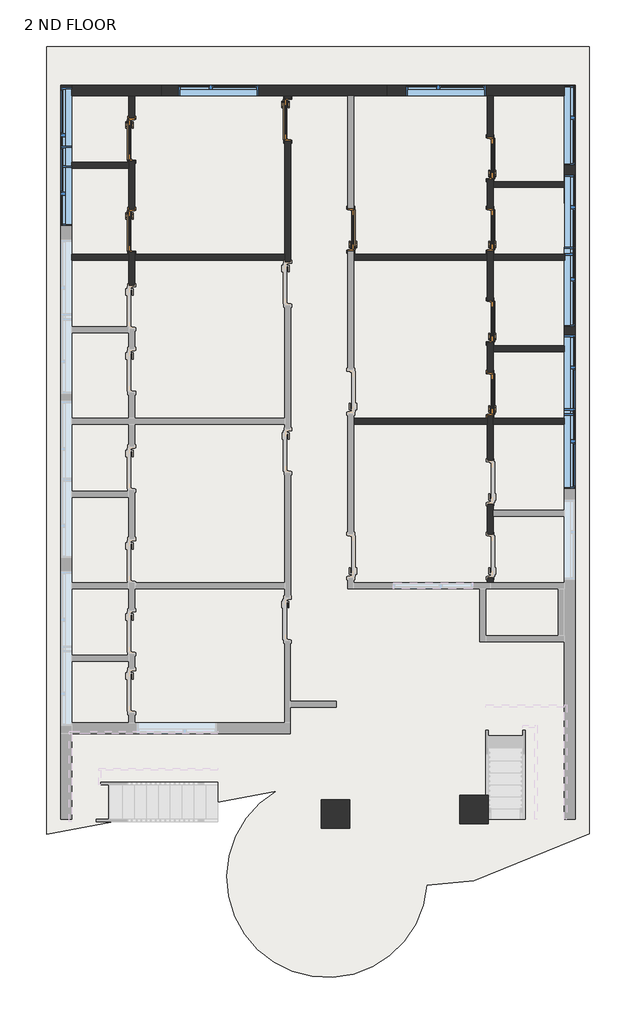
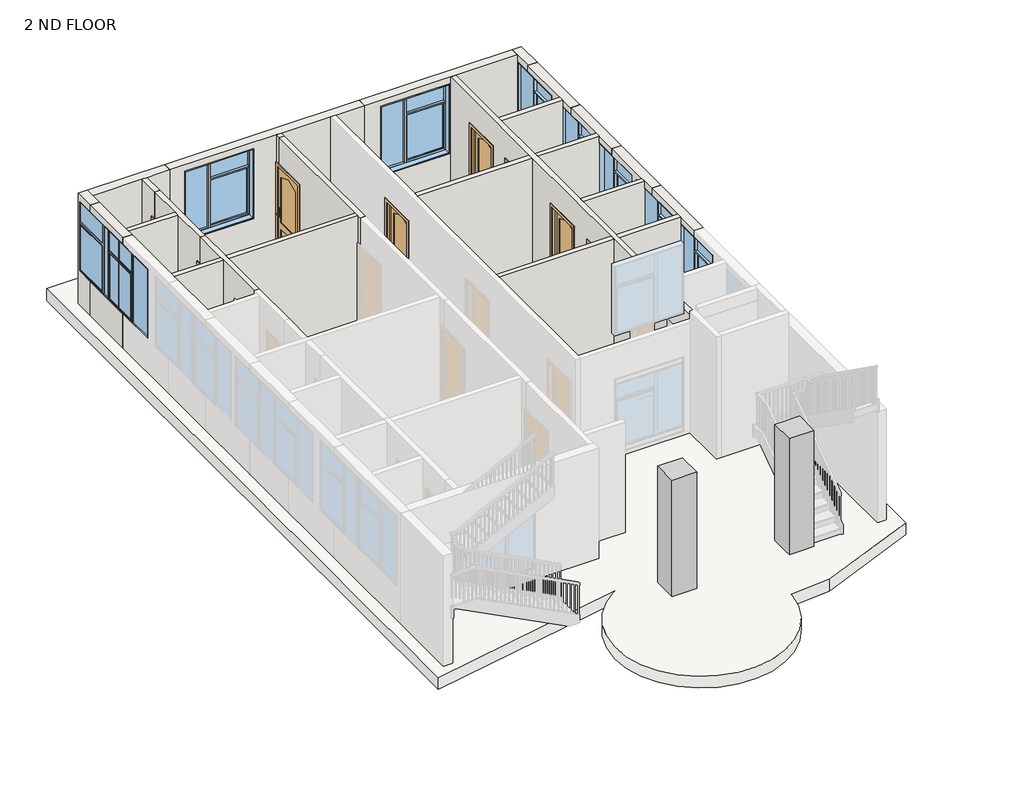
# One storey, part 2 of 4: 25 walls, 9 windows, 8 doors, 2 columns, 1 slab.
"""IFC4 building model written with IfcOpenShell, lengths in millimetres."""

from ifc_helpers import new_model, si_unit, point, frame, frame_2d, origin, place, context, project, spatial, polyline, circle_curve, trimmed, segment, composite_curve, outline, extrude, faceted_brep, transform, mapped, element, save
from components import column_ce31c9ba, door_346b4a94, m_window_casement_double_sidelight_1702_x_1829mm_c8b42c7f

model = new_model("IFC4")

# Units and contexts
model_context = context("Model", 3, world=origin())
ifc_project = project(units=[si_unit("LENGTHUNIT", "METRE", prefix="MILLI")], contexts=[model_context])

# Site, building, storey
site = spatial("IfcSite", under=ifc_project)
building = spatial("IfcBuilding", under=site)
storey = spatial("IfcBuildingStorey", under=building, Name="2 ND FLOOR", Elevation=6400.8)

# Columns
placement = place(None, origin())
element("IfcColumn", 1, ObjectType="Rectangular Column : 24\" x 24\"", at=placement, inside=storey, context=model_context, shape_type="SweptSolid", body=[
    extrude(outline(polyline([(2657.4891134, -7132.8082131), (2657.4891134, -7742.4082131), (2047.8891134, -7742.4082131), (2047.8891134, -7132.8082131), (2657.4891134, -7132.8082131)])), frame((0.0, 0.0, 6400.8), z_axis=(0.0, 0.0, 1.0), x_axis=(1.0, 0.0, 0.0)), (0.0, 0.0, 1.0), 3048.0),
])
column_shape = column_ce31c9ba(model_context)
element("IfcColumn", 2, ObjectType="Rectangular Column : 24\" x 24\"", at=placement, inside=storey, context=model_context, shape_type="MappedRepresentation", body=[
    mapped(column_shape, transform((-606.4108866, -7539.2082131, 0.0), x_axis=(1.0, 0.0, 0.0), y_axis=(0.0, 1.0, 0.0), z_axis=(0.0, 0.0, 1.0))),
])

# Doors
door_shape = door_346b4a94(model_context)
element("IfcDoor", 3, ObjectType="2'10\"X7'", at=placement, inside=storey, context=model_context, shape_type="MappedRepresentation", body=[
    mapped(door_shape, transform((2698.7641134, 6449.4399728, 6400.8), x_axis=(0.0, -1.0, 0.0), y_axis=(1.0, 0.0, 0.0), z_axis=(0.0, 0.0, 1.0))),
])
element("IfcDoor", 4, ObjectType="2'10\"X7'", at=placement, inside=storey, context=model_context, shape_type="MappedRepresentation", body=[
    mapped(door_shape, transform((2698.7641134, 4925.4399728, 6400.8), x_axis=(0.0, -1.0, 0.0), y_axis=(1.0, 0.0, 0.0), z_axis=(0.0, 0.0, 1.0))),
])
element("IfcDoor", 5, ObjectType="2'10\"X7'", at=placement, inside=storey, context=model_context, shape_type="MappedRepresentation", body=[
    mapped(door_shape, transform((2698.7641134, 2969.6399728, 6400.8), x_axis=(0.0, -1.0, 0.0), y_axis=(1.0, 0.0, 0.0), z_axis=(0.0, 0.0, 1.0))),
])
element("IfcDoor", 6, ObjectType="2'10\"X7'", at=placement, inside=storey, context=model_context, shape_type="MappedRepresentation", body=[
    mapped(door_shape, transform((2698.7641134, 1420.2399728, 6400.8), x_axis=(0.0, -1.0, 0.0), y_axis=(1.0, 0.0, 0.0), z_axis=(0.0, 0.0, 1.0))),
])
element("IfcDoor", 7, ObjectType="2'10\"X7'", at=placement, inside=storey, context=model_context, shape_type="MappedRepresentation", body=[
    mapped(door_shape, transform((-273.0358866, 4925.4399728, 6400.8), x_axis=(0.0, -1.0, 0.0), y_axis=(1.0, 0.0, 0.0), z_axis=(0.0, 0.0, 1.0))),
])
element("IfcDoor", 8, ObjectType="2'10\"X7'", at=placement, inside=storey, context=model_context, shape_type="MappedRepresentation", body=[
    mapped(door_shape, transform((-4952.9858866, 4900.320652, 6400.8), x_axis=(0.0, 1.0, 0.0), y_axis=(-1.0, 0.0, 0.0), z_axis=(0.0, 0.0, 1.0))),
])
element("IfcDoor", 9, ObjectType="2'10\"X7'", at=placement, inside=storey, context=model_context, shape_type="MappedRepresentation", body=[
    mapped(door_shape, transform((-4952.9858866, 6843.9929737, 6400.8), x_axis=(0.0, 1.0, 0.0), y_axis=(-1.0, 0.0, 0.0), z_axis=(0.0, 0.0, 1.0))),
])
element("IfcDoor", 10, ObjectType="2'10\"X7'", at=placement, inside=storey, context=model_context, shape_type="MappedRepresentation", body=[
    mapped(door_shape, transform((-1625.5858866, 7274.3310623, 6400.8), x_axis=(0.0, 1.0, 0.0), y_axis=(-1.0, 0.0, 0.0), z_axis=(0.0, 0.0, 1.0))),
])

# Slab
element("IfcSlab", 11, ObjectType="Generic - 12\"", at=placement, inside=storey, context=model_context, shape_type="SweptSolid", body=[
    extrude(outline(composite_curve([segment(polyline([(4815.1311655, 8833.6177996), (4815.1311655, -7955.7822004), (2347.1922936, -8966.8048135), (1347.7141783, -9054.247818)]), True, "CONTINUOUS"), segment(trimmed(circle_curve(frame_2d((-782.1411924, -8888.1832005)), 2136.3195821), [point((1347.7141783, -9054.247818))], [point((-1867.3559444, -7048.0282345))], False, "CARTESIAN"), True, "CONTINUOUS"), segment(polyline([(-1867.3559444, -7048.0282345), (-6765.9108866, -7971.0082131), (-6765.9108866, 8833.6177996), (4815.1311655, 8833.6177996)]), True, "CONTINUOUS")], self_intersect=False)), frame((0.0, 0.0, 6096.0), z_axis=(0.0, 0.0, 1.0), x_axis=(1.0, 0.0, 0.0)), (0.0, 0.0, 1.0), 304.8),
])

# Walls
element("IfcWall", 12, ObjectType="Generic - 4.5\"", at=placement, inside=storey, context=model_context, shape_type="SweptSolid", body=[
    extrude(outline(polyline([(7782.9399728, 9296.4), (7782.9399728, 6400.8), (7300.7929737, 6400.8), (7300.7929737, 8559.4), (7224.9929737, 8559.4), (7224.9929737, 9296.4), (7782.9399728, 9296.4)])), frame((-5013.3108866, 0.0, 0.0), z_axis=(1.0, 0.0, 0.0), x_axis=(0.0, 1.0, 0.0)), (0.0, 0.0, 1.0), 127.0),
])
element("IfcWall", 13, ObjectType="Generic - 4.5\"", at=placement, inside=storey, context=model_context, shape_type="Brep", body=[
    faceted_brep([(-5013.3108866, 5281.320652, 8559.4), (-5013.3108866, 5281.320652, 9296.4), (-5013.3108866, 6233.5399728, 9296.4), (-5013.3108866, 6360.5399728, 9296.4), (-5013.3108866, 7224.9929737, 9296.4), (-5013.3108866, 7224.9929737, 8559.4), (-5013.3108866, 6387.1929737, 8559.4), (-5013.3108866, 6387.1929737, 6400.8), (-5013.3108866, 6360.5399728, 6400.8), (-5013.3108866, 6233.5399728, 6400.8), (-5013.3108866, 5357.120652, 6400.8), (-5013.3108866, 5357.120652, 8559.4), (-4886.3108866, 5281.320652, 9296.4), (-4886.3108866, 5281.320652, 8559.4), (-4886.3108866, 5357.120652, 8559.4), (-4886.3108866, 5357.120652, 6400.8), (-4886.3108866, 6387.1929737, 6400.8), (-4886.3108866, 6387.1929737, 8559.4), (-4886.3108866, 7224.9929737, 8559.4), (-4886.3108866, 7224.9929737, 9296.4)], [[[0, 1, 2, 3, 4, 5, 6, 7, 8, 9, 10, 11]], [[12, 13, 14, 15, 16, 17, 18, 19]], [[15, 10, 9, 8, 7, 16]], [[1, 0, 13, 12]], [[4, 19, 18, 5]], [[14, 11, 10, 15]], [[11, 14, 13, 0]], [[17, 6, 5, 18]], [[6, 17, 16, 7]], [[4, 3, 2, 1, 12, 19]]]),
])
element("IfcWall", 14, ObjectType="Generic - 4.5\"", at=placement, inside=storey, context=model_context, shape_type="SweptSolid", body=[
    extrude(outline(polyline([(-5013.3108866, 6233.5399728), (-6232.5508078, 6233.5399728), (-6232.5508078, 6360.5399728), (-5013.3108866, 6360.5399728), (-5013.3108866, 6233.5399728)])), frame((0.0, 0.0, 6400.8), z_axis=(0.0, 0.0, 1.0), x_axis=(1.0, 0.0, 0.0)), (0.0, 0.0, 1.0), 2895.6),
])
element("IfcWall", 15, ObjectType="Generic - 4.5\"", at=placement, inside=storey, context=model_context, shape_type="SweptSolid", body=[
    extrude(outline(polyline([(-5013.3108866, 4277.7399728), (-6232.5508078, 4277.7399728), (-6232.5508078, 4404.7399728), (-5013.3108866, 4404.7399728), (-5013.3108866, 4277.7399728)])), frame((0.0, 0.0, 6400.8), z_axis=(0.0, 0.0, 1.0), x_axis=(1.0, 0.0, 0.0)), (0.0, 0.0, 1.0), 2895.6),
])
element("IfcWall", 16, ObjectType="Generic - 4.5\"", at=placement, inside=storey, context=model_context, shape_type="Brep", body=[
    faceted_brep([(-5013.3108866, 2968.8174518, 8559.4), (-5013.3108866, 2968.8174518, 9296.4), (-5013.3108866, 4277.7399728, 9296.4), (-5013.3108866, 4404.7399728, 9296.4), (-5013.3108866, 5281.320652, 9296.4), (-5013.3108866, 5281.320652, 8559.4), (-5013.3108866, 4443.520652, 8559.4), (-5013.3108866, 4443.520652, 6400.8), (-5013.3108866, 4404.7399728, 6400.8), (-5013.3108866, 4277.7399728, 6400.8), (-5013.3108866, 3730.4174518, 6400.8), (-5013.3108866, 3730.4174518, 8559.4), (-4886.3108866, 2968.8174518, 9296.4), (-4886.3108866, 2968.8174518, 8559.4), (-4886.3108866, 3730.4174518, 8559.4), (-4886.3108866, 3730.4174518, 6400.8), (-4886.3108866, 4277.7399728, 6400.8), (-4886.3108866, 4404.7399728, 6400.8), (-4886.3108866, 4443.520652, 6400.8), (-4886.3108866, 4443.520652, 8559.4), (-4886.3108866, 5281.320652, 8559.4), (-4886.3108866, 5281.320652, 9296.4), (-4886.3108866, 4404.7399728, 9296.4), (-4886.3108866, 4277.7399728, 9296.4)], [[[0, 1, 2, 3, 4, 5, 6, 7, 8, 9, 10, 11]], [[12, 13, 14, 15, 16, 17, 18, 19, 20, 21, 22, 23]], [[15, 10, 9, 8, 7, 18, 17, 16]], [[1, 0, 13, 12]], [[4, 21, 20, 5]], [[14, 11, 10, 15]], [[11, 14, 13, 0]], [[19, 6, 5, 20]], [[6, 19, 18, 7]], [[4, 3, 2, 1, 12, 23, 22, 21]]]),
])
element("IfcWall", 17, ObjectType="Generic - 4.5\"", at=placement, inside=storey, context=model_context, shape_type="SweptSolid", body=[
    extrude(outline(polyline([(-1685.9108866, 4277.7399728), (-4886.3108866, 4277.7399728), (-4886.3108866, 4404.7399728), (-1685.9108866, 4404.7399728), (-1685.9108866, 4277.7399728)])), frame((0.0, 0.0, 6400.8), z_axis=(0.0, 0.0, 1.0), x_axis=(1.0, 0.0, 0.0)), (0.0, 0.0, 1.0), 2895.6),
])
element("IfcWall", 18, ObjectType="Generic - 4.5\"", at=placement, inside=storey, context=model_context, shape_type="SweptSolid", body=[
    extrude(outline(polyline([(7782.9399728, 9296.4), (7782.9399728, 6400.8), (7731.1310623, 6400.8), (7731.1310623, 8559.4), (7655.3310623, 8559.4), (7655.3310623, 9296.4), (7782.9399728, 9296.4)])), frame((-1685.9108866, 0.0, 0.0), z_axis=(1.0, 0.0, 0.0), x_axis=(0.0, 1.0, 0.0)), (0.0, 0.0, 1.0), 127.0),
])
element("IfcWall", 19, ObjectType="Generic - 4.5\"", at=placement, inside=storey, context=model_context, shape_type="Brep", body=[
    faceted_brep([(-1685.9108866, 4182.2008884, 8559.4), (-1685.9108866, 4182.2008884, 9296.4), (-1685.9108866, 4277.7399728, 9296.4), (-1685.9108866, 4404.7399728, 9296.4), (-1685.9108866, 7655.3310623, 9296.4), (-1685.9108866, 7655.3310623, 8559.4), (-1685.9108866, 6817.5310623, 8559.4), (-1685.9108866, 6817.5310623, 6400.8), (-1685.9108866, 4404.7399728, 6400.8), (-1685.9108866, 4277.7399728, 6400.8), (-1685.9108866, 4232.6008884, 6400.8), (-1685.9108866, 4232.6008884, 8559.4), (-1558.9108866, 4182.2008884, 9296.4), (-1558.9108866, 4182.2008884, 8559.4), (-1558.9108866, 4232.6008884, 8559.4), (-1558.9108866, 4232.6008884, 6400.8), (-1558.9108866, 6817.5310623, 6400.8), (-1558.9108866, 6817.5310623, 8559.4), (-1558.9108866, 7655.3310623, 8559.4), (-1558.9108866, 7655.3310623, 9296.4), (-1685.4871817, 4182.2008884, 8559.4), (-1685.4871817, 4182.2008884, 9296.4)], [[[0, 1, 2, 3, 4, 5, 6, 7, 8, 9, 10, 11]], [[12, 13, 14, 15, 16, 17, 18, 19]], [[15, 10, 9, 8, 7, 16]], [[1, 0, 20, 13, 12, 21]], [[4, 19, 18, 5]], [[14, 11, 10, 15]], [[11, 14, 13, 20, 0]], [[17, 6, 5, 18]], [[6, 17, 16, 7]], [[4, 3, 2, 1, 21, 12, 19]]]),
])
element("IfcWall", 20, ObjectType="Generic - 4.5\"", at=placement, inside=storey, context=model_context, shape_type="Brep", body=[
    faceted_brep([(2632.0891134, 7782.9399728, 9296.4), (2632.0891134, 7782.9399728, 6400.8), (2632.0891134, 6906.2399728, 6400.8), (2632.0891134, 6906.2399728, 8559.4), (2632.0891134, 5992.6399728, 8559.4), (2632.0891134, 5992.6399728, 6400.8), (2632.0891134, 5382.2399728, 6400.8), (2632.0891134, 5382.2399728, 8559.4), (2632.0891134, 4468.6399728, 8559.4), (2632.0891134, 4468.6399728, 6400.8), (2632.0891134, 4404.7399728, 6400.8), (2632.0891134, 4277.7399728, 6400.8), (2632.0891134, 3426.4399728, 6400.8), (2632.0891134, 3426.4399728, 8559.4), (2632.0891134, 2512.8399728, 8559.4), (2632.0891134, 2512.8399728, 6400.8), (2632.0891134, 1877.0399728, 6400.8), (2632.0891134, 1877.0399728, 8559.4), (2632.0891134, 963.4399728, 8559.4), (2632.0891134, 963.4399728, 6400.8), (2632.0891134, 899.5399728, 6400.8), (2632.0891134, 772.5399728, 6400.8), (2632.0891134, -2.5600272, 6400.8), (2632.0891134, -2.5600272, 8559.4), (2632.0891134, -916.1600272, 8559.4), (2632.0891134, -916.1600272, 6400.8), (2632.0891134, -1577.3600272, 6400.8), (2632.0891134, -1577.3600272, 8559.4), (2632.0891134, -2490.9600272, 8559.4), (2632.0891134, -2490.9600272, 6400.8), (2632.0891134, -2605.6600272, 6400.8), (2632.0891134, -2605.6600272, 9296.4), (2632.0891134, 772.5399728, 9296.4), (2632.0891134, 899.5399728, 9296.4), (2632.0891134, 4277.7399728, 9296.4), (2632.0891134, 4404.7399728, 9296.4), (2759.0891134, 7782.9399728, 6400.8), (2759.0891134, 7782.9399728, 9296.4), (2759.0891134, 5954.1399728, 9296.4), (2759.0891134, 5827.1399728, 9296.4), (2759.0891134, 4404.7399728, 9296.4), (2759.0891134, 4277.7399728, 9296.4), (2759.0891134, 2448.9399728, 9296.4), (2759.0891134, 2321.9399728, 9296.4), (2759.0891134, 899.5399728, 9296.4), (2759.0891134, 772.5399728, 9296.4), (2759.0891134, -1056.2600272, 9296.4), (2759.0891134, -1183.2600272, 9296.4), (2759.0891134, -2605.6600272, 9296.4), (2759.0891134, -2605.6600272, 6400.8), (2759.0891134, -2490.9600272, 6400.8), (2759.0891134, -2490.9600272, 8559.4), (2759.0891134, -1577.3600272, 8559.4), (2759.0891134, -1577.3600272, 6400.8), (2759.0891134, -1183.2600272, 6400.8), (2759.0891134, -1056.2600272, 6400.8), (2759.0891134, -916.1600272, 6400.8), (2759.0891134, -916.1600272, 8559.4), (2759.0891134, -2.5600272, 8559.4), (2759.0891134, -2.5600272, 6400.8), (2759.0891134, 772.5399728, 6400.8), (2759.0891134, 899.5399728, 6400.8), (2759.0891134, 963.4399728, 6400.8), (2759.0891134, 963.4399728, 8559.4), (2759.0891134, 1877.0399728, 8559.4), (2759.0891134, 1877.0399728, 6400.8), (2759.0891134, 2321.9399728, 6400.8), (2759.0891134, 2448.9399728, 6400.8), (2759.0891134, 2512.8399728, 6400.8), (2759.0891134, 2512.8399728, 8559.4), (2759.0891134, 3426.4399728, 8559.4), (2759.0891134, 3426.4399728, 6400.8), (2759.0891134, 4277.7399728, 6400.8), (2759.0891134, 4404.7399728, 6400.8), (2759.0891134, 4468.6399728, 6400.8), (2759.0891134, 4468.6399728, 8559.4), (2759.0891134, 5382.2399728, 8559.4), (2759.0891134, 5382.2399728, 6400.8), (2759.0891134, 5827.1399728, 6400.8), (2759.0891134, 5954.1399728, 6400.8), (2759.0891134, 5992.6399728, 6400.8), (2759.0891134, 5992.6399728, 8559.4), (2759.0891134, 6906.2399728, 8559.4), (2759.0891134, 6906.2399728, 6400.8), (2695.5891134, -2605.6600272, 6400.8), (2695.5891134, -2605.6600272, 9296.4)], [[[0, 1, 2, 3, 4, 5, 6, 7, 8, 9, 10, 11, 12, 13, 14, 15, 16, 17, 18, 19, 20, 21, 22, 23, 24, 25, 26, 27, 28, 29, 30, 31, 32, 33, 34, 35]], [[36, 37, 38, 39, 40, 41, 42, 43, 44, 45, 46, 47, 48, 49, 50, 51, 52, 53, 54, 55, 56, 57, 58, 59, 60, 61, 62, 63, 64, 65, 66, 67, 68, 69, 70, 71, 72, 73, 74, 75, 76, 77, 78, 79, 80, 81, 82, 83]], [[1, 36, 83, 2]], [[5, 80, 79, 78, 77, 6]], [[9, 74, 73, 72, 71, 12, 11, 10]], [[15, 68, 67, 66, 65, 16]], [[19, 62, 61, 60, 59, 22, 21, 20]], [[25, 56, 55, 54, 53, 26]], [[49, 84, 30, 29, 50]], [[1, 0, 37, 36]], [[31, 30, 84, 49, 48, 85]], [[4, 81, 80, 5]], [[81, 4, 3, 82]], [[82, 3, 2, 83]], [[9, 8, 75, 74]], [[8, 7, 76, 75]], [[7, 6, 77, 76]], [[14, 69, 68, 15]], [[69, 14, 13, 70]], [[70, 13, 12, 71]], [[18, 63, 62, 19]], [[63, 18, 17, 64]], [[64, 17, 16, 65]], [[24, 57, 56, 25]], [[57, 24, 23, 58]], [[58, 23, 22, 59]], [[28, 51, 50, 29]], [[51, 28, 27, 52]], [[52, 27, 26, 53]], [[0, 35, 34, 33, 32, 31, 85, 48, 47, 46, 45, 44, 43, 42, 41, 40, 39, 38, 37]]]),
])
element("IfcWall", 21, ObjectType="Generic - 4.5\"", at=placement, inside=storey, context=model_context, shape_type="SweptSolid", body=[
    extrude(outline(polyline([(2632.0891134, 4277.7399728), (-212.7108866, 4277.7399728), (-212.7108866, 4404.7399728), (2632.0891134, 4404.7399728), (2632.0891134, 4277.7399728)])), frame((0.0, 0.0, 6400.8), z_axis=(0.0, 0.0, 1.0), x_axis=(1.0, 0.0, 0.0)), (0.0, 0.0, 1.0), 2895.6),
])
element("IfcWall", 22, ObjectType="Generic - 4.5\"", at=placement, inside=storey, context=model_context, shape_type="SweptSolid", body=[
    extrude(outline(polyline([(2632.0891134, 772.5399728), (-212.7108866, 772.5399728), (-212.7108866, 899.5399728), (2632.0891134, 899.5399728), (2632.0891134, 772.5399728)])), frame((0.0, 0.0, 6400.8), z_axis=(0.0, 0.0, 1.0), x_axis=(1.0, 0.0, 0.0)), (0.0, 0.0, 1.0), 2895.6),
])
element("IfcWall", 23, ObjectType="Generic - 4.5\"", at=placement, inside=storey, context=model_context, shape_type="SweptSolid", body=[
    extrude(outline(polyline([(4281.587404, 5827.1399728), (2759.0891134, 5827.1399728), (2759.0891134, 5954.1399728), (4281.587404, 5954.1399728), (4281.587404, 5827.1399728)])), frame((0.0, 0.0, 6400.8), z_axis=(0.0, 0.0, 1.0), x_axis=(1.0, 0.0, 0.0)), (0.0, 0.0, 1.0), 2895.6),
])
element("IfcWall", 24, ObjectType="Generic - 4.5\"", at=placement, inside=storey, context=model_context, shape_type="SweptSolid", body=[
    extrude(outline(polyline([(4283.9989713, 4277.7399728), (2759.0891134, 4277.7399728), (2759.0891134, 4404.7399728), (4283.9989713, 4404.7399728), (4283.9989713, 4277.7399728)])), frame((0.0, 0.0, 6400.8), z_axis=(0.0, 0.0, 1.0), x_axis=(1.0, 0.0, 0.0)), (0.0, 0.0, 1.0), 2895.6),
])
element("IfcWall", 25, ObjectType="Generic - 4.5\"", at=placement, inside=storey, context=model_context, shape_type="SweptSolid", body=[
    extrude(outline(polyline([(4281.0767915, 2321.9399728), (2759.0891134, 2321.9399728), (2759.0891134, 2448.9399728), (4281.0767915, 2448.9399728), (4281.0767915, 2321.9399728)])), frame((0.0, 0.0, 6400.8), z_axis=(0.0, 0.0, 1.0), x_axis=(1.0, 0.0, 0.0)), (0.0, 0.0, 1.0), 2895.6),
])
element("IfcWall", 26, ObjectType="Generic - 4.5\"", at=placement, inside=storey, context=model_context, shape_type="SweptSolid", body=[
    extrude(outline(polyline([(4283.0918814, 772.5399728), (2759.0891134, 772.5399728), (2759.0891134, 899.5399728), (4283.0918814, 899.5399728), (4283.0918814, 772.5399728)])), frame((0.0, 0.0, 6400.8), z_axis=(0.0, 0.0, 1.0), x_axis=(1.0, 0.0, 0.0)), (0.0, 0.0, 1.0), 2895.6),
])
element("IfcWall", 27, ObjectType="Generic - 9\"", at=placement, inside=storey, context=model_context, shape_type="Brep", body=[
    faceted_brep([(-6232.5108866, 7782.9399728, 6400.8), (-5013.3108866, 7782.9399728, 6400.8), (-4886.3108866, 7782.9399728, 6400.8), (-4318.2603585, 7782.9399728, 6400.8), (-4318.2603585, 7782.9399728, 9296.4), (-4886.3108866, 7782.9399728, 9296.4), (-5013.3108866, 7782.9399728, 9296.4), (-6232.5108866, 7782.9399728, 9296.4), (-6232.5108866, 8011.5399728, 6400.8), (-6232.5108866, 8011.5399728, 9296.4), (-4318.2603585, 8011.5399728, 9296.4), (-4318.2603585, 8011.5399728, 6400.8)], [[[0, 1, 2, 3, 4, 5, 6, 7]], [[8, 9, 10, 11]], [[3, 2, 1, 0, 8, 11]], [[4, 3, 11, 10]], [[0, 7, 9, 8]], [[7, 6, 5, 4, 10, 9]]]),
])
element("IfcWall", 28, ObjectType="Generic - 9\"", at=placement, inside=storey, context=model_context, shape_type="Brep", body=[
    faceted_brep([(-4318.2603585, 7782.9399728, 6400.8), (-1685.9108866, 7782.9399728, 6400.8), (-1558.9108866, 7782.9399728, 6400.8), (-339.7108866, 7782.9399728, 6400.8), (-212.7108866, 7782.9399728, 6400.8), (496.3553976, 7782.9399728, 6400.8), (496.3553976, 7782.9399728, 9296.4), (-212.7108866, 7782.9399728, 9296.4), (-339.7108866, 7782.9399728, 9296.4), (-1558.9108866, 7782.9399728, 9296.4), (-1685.9108866, 7782.9399728, 9296.4), (-4318.2603585, 7782.9399728, 9296.4), (-2248.1603585, 7782.9399728, 9129.6), (-2248.1603585, 7782.9399728, 7300.8), (-3949.9603585, 7782.9399728, 7300.8), (-3949.9603585, 7782.9399728, 9129.6), (-4318.2603585, 8011.5399728, 6400.8), (-4318.2603585, 8011.5399728, 9296.4), (496.3553976, 8011.5399728, 9296.4), (496.3553976, 8011.5399728, 6400.8), (-2248.1603585, 8011.5399728, 9129.6), (-3949.9603585, 8011.5399728, 9129.6), (-3949.9603585, 8011.5399728, 7300.8), (-2248.1603585, 8011.5399728, 7300.8)], [[[0, 1, 2, 3, 4, 5, 6, 7, 8, 9, 10, 11], [12, 13, 14, 15]], [[16, 17, 18, 19], [20, 21, 22, 23]], [[5, 4, 3, 2, 1, 0, 16, 19]], [[6, 5, 19, 18]], [[0, 11, 17, 16]], [[13, 12, 20, 23]], [[14, 13, 23, 22]], [[15, 14, 22, 21]], [[12, 15, 21, 20]], [[11, 10, 9, 8, 7, 6, 18, 17]]]),
])
element("IfcWall", 29, ObjectType="Generic - 9\"", at=placement, inside=storey, context=model_context, shape_type="Brep", body=[
    faceted_brep([(496.3553976, 7782.9399728, 6400.8), (2632.0891134, 7782.9399728, 6400.8), (2759.0891134, 7782.9399728, 6400.8), (4283.0891134, 7782.9399728, 6400.8), (4283.0891134, 7782.9399728, 9296.4), (2759.0891134, 7782.9399728, 9296.4), (2632.0891134, 7782.9399728, 9296.4), (496.3553976, 7782.9399728, 9296.4), (2606.6891134, 7782.9399728, 9129.6), (2606.6891134, 7782.9399728, 7300.8), (904.8891134, 7782.9399728, 7300.8), (904.8891134, 7782.9399728, 9129.6), (496.3553976, 8011.5399728, 6400.8), (496.3553976, 8011.5399728, 9296.4), (4283.0891134, 8011.5399728, 9296.4), (4283.0891134, 8011.5399728, 6400.8), (2606.6891134, 8011.5399728, 9129.6), (904.8891134, 8011.5399728, 9129.6), (904.8891134, 8011.5399728, 7300.8), (2606.6891134, 8011.5399728, 7300.8)], [[[0, 1, 2, 3, 4, 5, 6, 7], [8, 9, 10, 11]], [[12, 13, 14, 15], [16, 17, 18, 19]], [[3, 2, 1, 0, 12, 15]], [[0, 7, 13, 12]], [[9, 8, 16, 19]], [[10, 9, 19, 18]], [[11, 10, 18, 17]], [[8, 11, 17, 16]], [[4, 3, 15, 14]], [[7, 6, 5, 4, 14, 13]]]),
])
element("IfcWall", 30, ObjectType="Generic - 9\"", at=placement, inside=storey, context=model_context, shape_type="Brep", body=[
    faceted_brep([(4283.0891134, 8011.5399728, 6400.8), (4283.0891134, 7782.9399728, 6400.8), (4283.0891134, 7325.7399728, 6400.8), (4283.0891134, 7325.7399728, 7300.8), (4283.0891134, 7998.8399728, 7300.8), (4283.0891134, 7998.8399728, 9129.6), (4283.0891134, 7325.7399728, 9129.6), (4283.0891134, 7325.7399728, 9296.4), (4283.0891134, 7782.9399728, 9296.4), (4283.0891134, 8011.5399728, 9296.4), (4511.6891134, 7325.7399728, 6400.8), (4511.6891134, 8011.5399728, 6400.8), (4511.6891134, 8011.5399728, 9296.4), (4511.6891134, 7325.7399728, 9296.4), (4511.6891134, 7325.7399728, 9129.6), (4511.6891134, 7998.8399728, 9129.6), (4511.6891134, 7998.8399728, 7300.8), (4511.6891134, 7325.7399728, 7300.8), (4510.187404, 7325.7399728, 6400.8), (4510.187404, 7325.7399728, 7300.8), (4510.187404, 7325.7399728, 9296.4), (4510.187404, 7325.7399728, 9129.6)], [[[0, 1, 2, 3, 4, 5, 6, 7, 8, 9]], [[10, 11, 12, 13, 14, 15, 16, 17]], [[2, 1, 0, 11, 10, 18]], [[2, 18, 10, 17, 19, 3]], [[13, 20, 7, 6, 21, 14]], [[16, 4, 3, 19, 17]], [[4, 16, 15, 5]], [[5, 15, 14, 21, 6]], [[0, 9, 12, 11]], [[9, 8, 7, 20, 13, 12]]]),
])
element("IfcWall", 31, ObjectType="Generic - 9\"", at=placement, inside=storey, context=model_context, shape_type="Brep", body=[
    faceted_brep([(4281.587404, 7325.7399728, 6400.8), (4281.587404, 5954.1399728, 6400.8), (4281.587404, 5827.1399728, 6400.8), (4281.587404, 5490.9915892, 6400.8), (4281.587404, 5490.9915892, 7300.8), (4281.587404, 6087.8915892, 7300.8), (4281.587404, 6087.8915892, 9129.6), (4281.587404, 5490.9915892, 9129.6), (4281.587404, 5490.9915892, 9296.4), (4281.587404, 5827.1399728, 9296.4), (4281.587404, 5954.1399728, 9296.4), (4281.587404, 7325.7399728, 9296.4), (4281.587404, 7325.7399728, 9129.6), (4281.587404, 6297.0399728, 9129.6), (4281.587404, 6297.0399728, 7300.8), (4281.587404, 7325.7399728, 7300.8), (4510.187404, 5490.9915892, 6400.8), (4510.187404, 7325.7399728, 6400.8), (4510.187404, 7325.7399728, 7300.8), (4510.187404, 6297.0399728, 7300.8), (4510.187404, 6297.0399728, 9129.6), (4510.187404, 7325.7399728, 9129.6), (4510.187404, 7325.7399728, 9296.4), (4510.187404, 5490.9915892, 9296.4), (4510.187404, 5490.9915892, 9129.6), (4510.187404, 6087.8915892, 9129.6), (4510.187404, 6087.8915892, 7300.8), (4510.187404, 5490.9915892, 7300.8), (4283.0891134, 7325.7399728, 6400.8), (4283.9989713, 5490.9915892, 6400.8), (4283.9989713, 5490.9915892, 7300.8), (4283.9989713, 5490.9915892, 9296.4), (4283.9989713, 5490.9915892, 9129.6), (4283.0891134, 7325.7399728, 7300.8), (4283.0891134, 7325.7399728, 9296.4), (4283.0891134, 7325.7399728, 9129.6)], [[[0, 1, 2, 3, 4, 5, 6, 7, 8, 9, 10, 11, 12, 13, 14, 15]], [[16, 17, 18, 19, 20, 21, 22, 23, 24, 25, 26, 27]], [[3, 2, 1, 0, 28, 17, 16, 29]], [[3, 29, 16, 27, 30, 4]], [[23, 31, 8, 7, 32, 24]], [[17, 28, 0, 15, 33, 18]], [[12, 11, 34, 22, 21, 35]], [[13, 20, 19, 14]], [[14, 19, 18, 33, 15]], [[20, 13, 12, 35, 21]], [[26, 5, 4, 30, 27]], [[5, 26, 25, 6]], [[6, 25, 24, 32, 7]], [[11, 10, 9, 8, 31, 23, 22, 34]]]),
])
element("IfcWall", 32, ObjectType="Generic - 9\"", at=placement, inside=storey, context=model_context, shape_type="Brep", body=[
    faceted_brep([(4283.9989713, 5490.9915892, 6400.8), (4283.9989713, 4404.7399728, 6400.8), (4283.9989713, 4277.7399728, 6400.8), (4283.9989713, 3730.8359967, 6400.8), (4283.9989713, 3730.8359967, 7300.8), (4283.9989713, 5490.9915892, 7300.8), (4512.5989713, 3730.8359967, 6400.8), (4512.5989713, 5490.9915892, 6400.8), (4512.5989713, 5490.9915892, 7300.8), (4512.5989713, 3730.8359967, 7300.8), (4510.187404, 5490.9915892, 6400.8), (4509.6767915, 3730.8359967, 6400.8), (4509.6767915, 3730.8359967, 7300.8), (4510.187404, 5490.9915892, 7300.8)], [[[0, 1, 2, 3, 4, 5]], [[6, 7, 8, 9]], [[3, 2, 1, 0, 10, 7, 6, 11]], [[3, 11, 6, 9, 12, 4]], [[7, 10, 0, 5, 13, 8]], [[8, 13, 5, 4, 12, 9]]]),
    faceted_brep([(4283.9989713, 5490.9915892, 9296.4), (4283.9989713, 5490.9915892, 9129.6), (4283.9989713, 3730.8359967, 9129.6), (4283.9989713, 3730.8359967, 9296.4), (4283.9989713, 4277.7399728, 9296.4), (4283.9989713, 4404.7399728, 9296.4), (4512.5989713, 3730.8359967, 9129.6), (4512.5989713, 5490.9915892, 9129.6), (4512.5989713, 5490.9915892, 9296.4), (4512.5989713, 3730.8359967, 9296.4), (4509.6767915, 3730.8359967, 9296.4), (4509.6767915, 3730.8359967, 9129.6), (4510.187404, 5490.9915892, 9296.4), (4510.187404, 5490.9915892, 9129.6)], [[[0, 1, 2, 3, 4, 5]], [[6, 7, 8, 9]], [[9, 10, 3, 2, 11, 6]], [[1, 0, 12, 8, 7, 13]], [[1, 13, 7, 6, 11, 2]], [[0, 5, 4, 3, 10, 9, 8, 12]]]),
])
element("IfcWall", 33, ObjectType="Generic - 9\"", at=placement, inside=storey, context=model_context, shape_type="Brep", body=[
    faceted_brep([(4281.0767915, 3730.8359967, 6400.8), (4281.0767915, 2448.9399728, 6400.8), (4281.0767915, 2321.9399728, 6400.8), (4281.0767915, 2023.9001312, 6400.8), (4281.0767915, 2023.9001312, 7300.8), (4281.0767915, 2671.6001312, 7300.8), (4281.0767915, 2671.6001312, 9129.6), (4281.0767915, 2023.9001312, 9129.6), (4281.0767915, 2023.9001312, 9296.4), (4281.0767915, 2321.9399728, 9296.4), (4281.0767915, 2448.9399728, 9296.4), (4281.0767915, 3730.8359967, 9296.4), (4281.0767915, 3730.8359967, 9129.6), (4281.0767915, 2854.5359967, 9129.6), (4281.0767915, 2854.5359967, 7300.8), (4281.0767915, 3730.8359967, 7300.8), (4509.6767915, 2023.9001312, 6400.8), (4509.6767915, 3730.8359967, 6400.8), (4509.6767915, 3730.8359967, 7300.8), (4509.6767915, 2854.5359967, 7300.8), (4509.6767915, 2854.5359967, 9129.6), (4509.6767915, 3730.8359967, 9129.6), (4509.6767915, 3730.8359967, 9296.4), (4509.6767915, 2023.9001312, 9296.4), (4509.6767915, 2023.9001312, 9129.6), (4509.6767915, 2671.6001312, 9129.6), (4509.6767915, 2671.6001312, 7300.8), (4509.6767915, 2023.9001312, 7300.8), (4283.9989713, 3730.8359967, 6400.8), (4283.0918814, 2023.9001312, 6400.8), (4283.0918814, 2023.9001312, 7300.8), (4283.0918814, 2023.9001312, 9296.4), (4283.0918814, 2023.9001312, 9129.6), (4283.9989713, 3730.8359967, 7300.8), (4283.9989713, 3730.8359967, 9296.4), (4283.9989713, 3730.8359967, 9129.6)], [[[0, 1, 2, 3, 4, 5, 6, 7, 8, 9, 10, 11, 12, 13, 14, 15]], [[16, 17, 18, 19, 20, 21, 22, 23, 24, 25, 26, 27]], [[3, 2, 1, 0, 28, 17, 16, 29]], [[3, 29, 16, 27, 30, 4]], [[23, 31, 8, 7, 32, 24]], [[17, 28, 0, 15, 33, 18]], [[12, 11, 34, 22, 21, 35]], [[13, 20, 19, 14]], [[14, 19, 18, 33, 15]], [[20, 13, 12, 35, 21]], [[26, 5, 4, 30, 27]], [[5, 26, 25, 6]], [[6, 25, 24, 32, 7]], [[11, 10, 9, 8, 31, 23, 22, 34]]]),
])
element("IfcWall", 34, ObjectType="Generic - 9\"", at=placement, inside=storey, context=model_context, shape_type="Brep", body=[
    faceted_brep([(4283.0918814, 2023.9001312, 6400.8), (4283.0918814, 899.5399728, 6400.8), (4283.0918814, 772.5399728, 6400.8), (4283.0918814, 200.5184135, 6400.8), (4283.0918814, 200.5184135, 7300.8), (4283.0918814, 2023.9001312, 7300.8), (4511.6918814, 200.5184135, 6400.8), (4511.6918814, 2023.9001312, 6400.8), (4511.6918814, 2023.9001312, 7300.8), (4511.6918814, 200.5184135, 7300.8), (4509.6767915, 2023.9001312, 6400.8), (4510.3311655, 200.5184135, 6400.8), (4510.3311655, 200.5184135, 7300.8), (4509.6767915, 2023.9001312, 7300.8)], [[[0, 1, 2, 3, 4, 5]], [[6, 7, 8, 9]], [[3, 2, 1, 0, 10, 7, 6, 11]], [[3, 11, 6, 9, 12, 4]], [[7, 10, 0, 5, 13, 8]], [[8, 13, 5, 4, 12, 9]]]),
    faceted_brep([(4283.0918814, 2023.9001312, 9296.4), (4283.0918814, 2023.9001312, 9129.6), (4283.0918814, 200.5184135, 9129.6), (4283.0918814, 200.5184135, 9296.4), (4283.0918814, 772.5399728, 9296.4), (4283.0918814, 899.5399728, 9296.4), (4511.6918814, 200.5184135, 9129.6), (4511.6918814, 2023.9001312, 9129.6), (4511.6918814, 2023.9001312, 9296.4), (4511.6918814, 200.5184135, 9296.4), (4510.3311655, 200.5184135, 9296.4), (4510.3311655, 200.5184135, 9129.6), (4509.6767915, 2023.9001312, 9296.4), (4509.6767915, 2023.9001312, 9129.6)], [[[0, 1, 2, 3, 4, 5]], [[6, 7, 8, 9]], [[9, 10, 3, 2, 11, 6]], [[1, 0, 12, 8, 7, 13]], [[1, 13, 7, 6, 11, 2]], [[0, 5, 4, 3, 10, 9, 8, 12]]]),
])
element("IfcWall", 35, ObjectType="Generic - 9\"", at=placement, inside=storey, context=model_context, shape_type="Brep", body=[
    faceted_brep([(-6232.5508078, 6088.0863192, 6400.8), (-6232.5508078, 6233.5399728, 6400.8), (-6232.5508078, 6360.5399728, 6400.8), (-6232.5508078, 7490.3748838, 6400.8), (-6232.5508078, 7490.3748838, 7300.8), (-6232.5508078, 6088.0863192, 7300.8), (-6461.1508078, 7490.3748838, 6400.8), (-6461.1508078, 6088.0863192, 6400.8), (-6461.1508078, 6088.0863192, 7300.8), (-6461.1508078, 7490.3748838, 7300.8)], [[[0, 1, 2, 3, 4, 5]], [[6, 7, 8, 9]], [[3, 2, 1, 0, 7, 6]], [[3, 6, 9, 4]], [[7, 0, 5, 8]], [[4, 9, 8, 5]]]),
    faceted_brep([(-6232.5508078, 6088.0863192, 9129.6), (-6232.5508078, 7490.3748838, 9129.6), (-6232.5508078, 7490.3748838, 9296.4), (-6232.5508078, 6360.5399728, 9296.4), (-6232.5508078, 6233.5399728, 9296.4), (-6232.5508078, 6088.0863192, 9296.4), (-6461.1508078, 7490.3748838, 9296.4), (-6461.1508078, 7490.3748838, 9129.6), (-6461.1508078, 6088.0863192, 9129.6), (-6461.1508078, 6088.0863192, 9296.4)], [[[0, 1, 2, 3, 4, 5]], [[6, 7, 8, 9]], [[2, 1, 7, 6]], [[5, 9, 8, 0]], [[7, 1, 0, 8]], [[5, 4, 3, 2, 6, 9]]]),
])
element("IfcWall", 36, ObjectType="Generic - 9\"", at=placement, inside=storey, context=model_context, shape_type="Brep", body=[
    faceted_brep([(-6232.5108866, 7490.3748838, 6400.8), (-6232.5108866, 7782.9399728, 6400.8), (-6232.5108866, 8011.5399728, 6400.8), (-6232.5108866, 8011.5399728, 9296.4), (-6232.5108866, 7782.9399728, 9296.4), (-6232.5108866, 7490.3748838, 9296.4), (-6232.5108866, 7490.3748838, 9129.6), (-6232.5108866, 7960.2748838, 9129.6), (-6232.5108866, 7960.2748838, 7300.8), (-6232.5108866, 7490.3748838, 7300.8), (-6461.1108866, 8011.5399728, 6400.8), (-6461.1108866, 7490.3748838, 6400.8), (-6461.1108866, 7490.3748838, 7300.8), (-6461.1108866, 7960.2748838, 7300.8), (-6461.1108866, 7960.2748838, 9129.6), (-6461.1108866, 7490.3748838, 9129.6), (-6461.1108866, 7490.3748838, 9296.4), (-6461.1108866, 8011.5399728, 9296.4)], [[[0, 1, 2, 3, 4, 5, 6, 7, 8, 9]], [[10, 11, 12, 13, 14, 15, 16, 17]], [[2, 1, 0, 11, 10]], [[11, 0, 9, 12]], [[5, 16, 15, 6]], [[7, 14, 13, 8]], [[8, 13, 12, 9]], [[14, 7, 6, 15]], [[3, 2, 10, 17]], [[5, 4, 3, 17, 16]]]),
])

# Windows
m_window_casement_double_sidelight_1702_x_1829mm_shape = m_window_casement_double_sidelight_1702_x_1829mm_c8b42c7f(model_context)
element("IfcWindow", 37, ObjectType="M_Window-Casement-Double-Sidelight : 1702 x 1829mm", at=placement, inside=storey, context=model_context, shape_type="MappedRepresentation", body=[
    mapped(m_window_casement_double_sidelight_1702_x_1829mm_shape, transform((-6346.8508078, 7109.3748838, 6400.8), x_axis=(0.0, 1.0, 0.0), y_axis=(-1.0, 0.0, 0.0), z_axis=(0.0, 0.0, 1.0))),
])
element("IfcWindow", 38, ObjectType="M_Window-Casement-Double-Sidelight : 1702 x 1829mm", at=placement, inside=storey, context=model_context, shape_type="MappedRepresentation", body=[
    mapped(m_window_casement_double_sidelight_1702_x_1829mm_shape, transform((-6346.8508078, 5859.4863192, 6400.8), x_axis=(0.0, 1.0, 0.0), y_axis=(-1.0, 0.0, 0.0), z_axis=(0.0, 0.0, 1.0))),
])
element("IfcWindow", 39, ObjectType="M_Window-Casement-Double-Sidelight : 1702 x 1829mm", at=placement, inside=storey, context=model_context, shape_type="MappedRepresentation", body=[
    mapped(m_window_casement_double_sidelight_1702_x_1829mm_shape, transform((4395.887404, 7147.9399728, 6400.8), x_axis=(0.0, -1.0, 0.0), y_axis=(1.0, 0.0, 0.0), z_axis=(0.0, 0.0, 1.0))),
])
element("IfcWindow", 40, ObjectType="M_Window-Casement-Double-Sidelight : 1702 x 1829mm", at=placement, inside=storey, context=model_context, shape_type="MappedRepresentation", body=[
    mapped(m_window_casement_double_sidelight_1702_x_1829mm_shape, transform((4398.2989713, 5236.9915892, 6400.8), x_axis=(0.0, -1.0, 0.0), y_axis=(1.0, 0.0, 0.0), z_axis=(0.0, 0.0, 1.0))),
])
element("IfcWindow", 41, ObjectType="M_Window-Casement-Double-Sidelight : 1702 x 1829mm", at=placement, inside=storey, context=model_context, shape_type="MappedRepresentation", body=[
    mapped(m_window_casement_double_sidelight_1702_x_1829mm_shape, transform((4395.3767915, 3705.4359967, 6400.8), x_axis=(0.0, -1.0, 0.0), y_axis=(1.0, 0.0, 0.0), z_axis=(0.0, 0.0, 1.0))),
])
element("IfcWindow", 42, ObjectType="M_Window-Casement-Double-Sidelight : 1702 x 1829mm", at=placement, inside=storey, context=model_context, shape_type="MappedRepresentation", body=[
    mapped(m_window_casement_double_sidelight_1702_x_1829mm_shape, transform((4397.3918814, 1820.7001312, 6400.8), x_axis=(0.0, -1.0, 0.0), y_axis=(1.0, 0.0, 0.0), z_axis=(0.0, 0.0, 1.0))),
])
element("IfcWindow", 43, ObjectType="M_Window-Casement-Double-Sidelight : 1702 x 1829mm", at=placement, inside=storey, context=model_context, shape_type="MappedRepresentation", body=[
    mapped(m_window_casement_double_sidelight_1702_x_1829mm_shape, transform((4396.0311655, 251.8399728, 6400.8), x_axis=(0.0, -1.0, 0.0), y_axis=(1.0, 0.0, 0.0), z_axis=(0.0, 0.0, 1.0))),
])
element("IfcWindow", 44, ObjectType="M_Window-Casement-Double-Sidelight : 1702 x 1829mm", at=placement, inside=storey, context=model_context, shape_type="MappedRepresentation", body=[
    mapped(m_window_casement_double_sidelight_1702_x_1829mm_shape, transform((-3099.0603585, 7897.2399728, 6400.8), x_axis=(1.0, 0.0, 0.0), y_axis=(0.0, 1.0, 0.0), z_axis=(0.0, 0.0, 1.0))),
])
element("IfcWindow", 45, ObjectType="M_Window-Casement-Double-Sidelight : 1702 x 1829mm", at=placement, inside=storey, context=model_context, shape_type="MappedRepresentation", body=[
    mapped(m_window_casement_double_sidelight_1702_x_1829mm_shape, transform((1755.7891134, 7897.2399728, 6400.8), x_axis=(1.0, 0.0, 0.0), y_axis=(0.0, 1.0, 0.0), z_axis=(0.0, 0.0, 1.0))),
])

save(model, "model.ifc")

# Revit data of these elements
# Type "Rectangular Column : 24\" x 24\""
#   Assembly Code = "B1010200"
#   Depth = 2' - 0"
#   Offset Base = 0' - 0"
#   Offset Top = 0' - 0"
#   Width = 2' - 0"
#   Material = none
# Type "2'10\"X7'"
#   Type Mark = "9"
#   Assembly Code = "B2030100"
#   Analytic Construction = "French door, wood frame with single glass"
#   Threshold Offset [instance default] = 0' - 0.59055"
#   Thickness = 0' - 1.37795"
#   Thermal Resistance (R) = 1.0696 (h·ft²·°F)/BTU
#   Swing Angle [instance default] = 90.00°
#   Stiles = 0' - 4.72441"
#   Rough Width = 2' - 11.9685"
#   Rough Height = 7' - 0.98425"
#   Radius = 1' - 5.56901"
#   Lock Rail = 0' - 7.08661"
#   Height = 7' - 0"
#   Width = 2' - 10"
#   Heat Transfer Coefficient (U) = 0.9350 BTU/(h·ft²·°F)
#   Door Offset [instance default] = 0' - 0"
#   Bottom Rail = 0' - 9.44882"
#   Threshold [instance default] = yes
#   Function = 1
#   Exterior Trim [instance default] = yes
#   Trim Material = Cherry
#   Threshold Material = Cherry
#   Panel Material = Cherry
#   Glazing = Glass
#   Frame Material = Cherry
#   Door Handle Material = Aluminum
#   Visual Light Transmittance = 0
#   Solar Heat Gain Coefficient = 0
#   Wall Closure = (empty or 0)
#   Construction Type = (empty or 0)
# Type "Generic - 12\""
#   Assembly Code = "B1010"
#   Function = 0
#   Layers, outside or top first: 1' - 0" no material (function 1)
# Type "Generic - 4.5\""
#   Assembly Code = "B2010"
#   Layers, outside or top first: 0' - 5" no material (function 1)
# Type "Generic - 9\""
#   Assembly Code = "B2010"
#   Layers, outside or top first: 0' - 9" no material (function 1)
# Type "M_Window-Casement-Double-Sidelight : 1702 x 1829mm"
#   Type Mark = "18"
#   Fire Rating = "0.5h"
#   Assembly Code = "B2020100"
#   Analytic Construction = "Double glazing - domestic"
#   Window Inset [instance default] = 0' - 0.62598"
#   Wall Thickness [instance default] = 0' - 5.90551"
#   Visual Light Transmittance = 0.81
#   Transom Height Ratio = 0.3
#   Transom Height = 1' - 9.6"
#   Thermal Resistance (R) = 1.8146 (h·ft²·°F)/BTU
#   Solar Heat Gain Coefficient = 0.76
#   Side Width = 2' - 2.8"
#   Rough Width = 5' - 7.59055"
#   Rough Height = 6' - 0.59055"
#   Opening Window Width = 3' - 4.2"
#   Opening Window Height = 4' - 2.4"
#   Heat Transfer Coefficient (U) = 0.5511 BTU/(h·ft²·°F)
#   Height = 6' - 0"
#   Frame Gap 3 [instance default] = 0' - 1.65041"
#   Frame Gap 2 [instance default] = 0' - 0.62598"
#   Frame Gap 1 = 0' - 1 51/128"
#   Default Sill Height = 2' - 11.43307"
#   Width = 5' - 7"
#   Frame Material = Metal - Aluminum
#   Glass Panel Material = Glass
#   Wall Closure = (empty or 0)
# Elements 1, 2 (IfcColumn, "Rectangular Column : 24\" x 24\"")
#   Phase Created = New Construction
# Elements 3, 4, 5, 6, 7, 8, 9, 10 (IfcDoor, "2'10\"X7'")
#   Threshold Offset = 0' - 0.59055"
#   Swing Angle = 90.00°
#   Door Offset = 0' - 0"
#   Threshold = yes
#   Exterior Trim = yes
#   Phase Created = New Construction
#   Materials on its faces: "Cherry", "Aluminum", "Glass"
# Element 11 (IfcSlab, "Generic - 12\"")
#   Height Offset From Level = 0' - 0"
#   Phase Created = New Construction
#   Materials on its faces: "Default Floor"
# Elements 12, 13, 14, 15, 16, 17, 18, 19, 20, 21, 22, 23, 24, 25, 26 (IfcWall, "Generic - 4.5\"")
#   Top Offset = 0' - 0"
#   Base Offset = 0' - 0"
#   wall height = 9' - 6"
#   Phase Created = New Construction
#   Base Constraint = 2 ND FLOOR
#   Top Constraint = 3 RD FLOOR
#   Materials on its faces: "Default Wall"
# Elements 27, 31, 35, 36 (IfcWall, "Generic - 9\"")
#   Top Offset = 0' - 0"
#   Base Offset = 0' - 0"
#   wall height = 9' - 6"
#   Phase Created = New Construction
#   Base Constraint = 2 ND FLOOR
#   Top Constraint = 3 RD FLOOR
#   Materials on its faces: "Default Wall"
# Elements 28, 29, 30, 32, 33, 34 (IfcWall, "Generic - 9\"")
#   Top Offset = -0' - 6"
#   Base Offset = 0' - 0"
#   wall height = 9' - 6"
#   Phase Created = New Construction
#   Base Constraint = 2 ND FLOOR
#   Top Constraint = 3 RD FLOOR
#   Materials on its faces: "Default Wall"
# Element 37 (IfcWindow, "M_Window-Casement-Double-Sidelight : 1702 x 1829mm")
#   Mark = "33"
#   Window Inset = 0' - 0.62598"
#   Frame Gap 3 = 0' - 1.65041"
#   Frame Gap 2 = 0' - 0.62598"
#   Phase Created = New Construction
#   Materials on its faces: "Metal - Aluminum", "Glass"
# Element 38 (IfcWindow, "M_Window-Casement-Double-Sidelight : 1702 x 1829mm")
#   Mark = "34"
#   Window Inset = 0' - 0.62598"
#   Frame Gap 3 = 0' - 1.65041"
#   Frame Gap 2 = 0' - 0.62598"
#   Phase Created = New Construction
#   Materials on its faces: "Metal - Aluminum", "Glass"
# Element 39 (IfcWindow, "M_Window-Casement-Double-Sidelight : 1702 x 1829mm")
#   Mark = "41"
#   Window Inset = 0' - 0.62598"
#   Frame Gap 3 = 0' - 1.65041"
#   Frame Gap 2 = 0' - 0.62598"
#   Phase Created = New Construction
#   Materials on its faces: "Metal - Aluminum", "Glass"
# Element 40 (IfcWindow, "M_Window-Casement-Double-Sidelight : 1702 x 1829mm")
#   Mark = "42"
#   Window Inset = 0' - 0.62598"
#   Frame Gap 3 = 0' - 1.65041"
#   Frame Gap 2 = 0' - 0.62598"
#   Phase Created = New Construction
#   Materials on its faces: "Metal - Aluminum", "Glass"
# Element 41 (IfcWindow, "M_Window-Casement-Double-Sidelight : 1702 x 1829mm")
#   Mark = "43"
#   Window Inset = 0' - 0.62598"
#   Frame Gap 3 = 0' - 1.65041"
#   Frame Gap 2 = 0' - 0.62598"
#   Phase Created = New Construction
#   Materials on its faces: "Metal - Aluminum", "Glass"
# Element 42 (IfcWindow, "M_Window-Casement-Double-Sidelight : 1702 x 1829mm")
#   Mark = "44"
#   Window Inset = 0' - 0.62598"
#   Frame Gap 3 = 0' - 1.65041"
#   Frame Gap 2 = 0' - 0.62598"
#   Phase Created = New Construction
#   Materials on its faces: "Metal - Aluminum", "Glass"
# Element 43 (IfcWindow, "M_Window-Casement-Double-Sidelight : 1702 x 1829mm")
#   Mark = "45"
#   Window Inset = 0' - 0.62598"
#   Frame Gap 3 = 0' - 1.65041"
#   Frame Gap 2 = 0' - 0.62598"
#   Phase Created = New Construction
#   Materials on its faces: "Metal - Aluminum", "Glass"
# Element 44 (IfcWindow, "M_Window-Casement-Double-Sidelight : 1702 x 1829mm")
#   Mark = "47"
#   Window Inset = 0' - 0.62598"
#   Frame Gap 3 = 0' - 1.65041"
#   Frame Gap 2 = 0' - 0.62598"
#   Phase Created = New Construction
#   Materials on its faces: "Metal - Aluminum", "Glass"
# Element 45 (IfcWindow, "M_Window-Casement-Double-Sidelight : 1702 x 1829mm")
#   Mark = "48"
#   Window Inset = 0' - 0.62598"
#   Frame Gap 3 = 0' - 1.65041"
#   Frame Gap 2 = 0' - 0.62598"
#   Phase Created = New Construction
#   Materials on its faces: "Metal - Aluminum", "Glass"
# Materials
#   "Cherry": class "Wood", colour RGB 226 177 128, transparency 0, Description = "Prunus Serotina", Cost = 0
#   "Glass": class "Glass", colour RGB 0 128 192, transparency 0.75, Description = "Soda Lime Glass", Cost = 0
#   "Aluminum": class "Metal", colour RGB 247 247 247, transparency 0, Description = "Aluminum 6061", Cost = 0
#   "Metal - Aluminum": class "Metal", colour RGB 247 247 247, transparency 0
#   "Default Floor": colour RGB 128 128 128, transparency 0, Cost = 0
#   "Default Wall": colour RGB 128 128 128, transparency 0, Cost = 0
